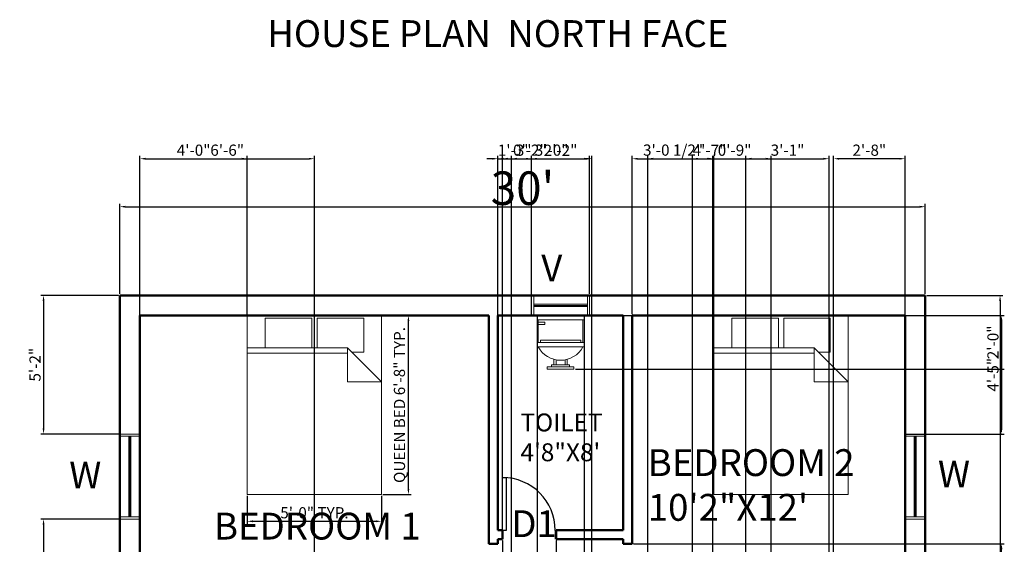
# Model space of a CAD drawing. Units: inches. Extents: x 2050 to 2529, y 1266 to 1968.
# Tile 5 of 5: x 2050 to 2490, y 1733 to 1968. Entities that reach past the tile are written whole.
import ezdxf

# ---------------------------------------------------------------- set-up
doc = ezdxf.new("R2010")
doc.units = ezdxf.units.IN
for name, color, linetype, lineweight in [('A-ANNO-DIMS', 2, 'Continuous', 18), ('A-ANNO-TEXT', 7, 'Continuous', 18), ('A-AREA-IDEN', 7, 'Continuous', 25), ('A-DOOR', 3, 'Continuous', 25), ('A-FLOR-FIXT', 9, 'Continuous', 18), ('A-FURN', 8, 'Continuous', 18), ('A-GLAZ', 4, 'Continuous', 18), ('A-WALL', 7, 'Continuous', 50)]:
    doc.layers.add(name, color=color, linetype=linetype, lineweight=lineweight)
doc.styles.get("Standard").update_dxf_attribs({"font": 'arial.ttf'})
doc.dimstyles.new('ISO-25', dxfattribs={"dimtxt": 5, "dimasz": 2.5, "dimexe": 1.25, "dimexo": 0.625, "dimtad": 1, "dimlunit": 3, "dimtxsty": 'Standard', "dimcen": 2.5, "dimadec": 0, "dimazin": 0, "dimtfac": 1, "dimtmove": 0, "dimatfit": 3, "dimfxl": 1, "dimarcsym": 0})

# ---------------------------------------------------------------- blocks, each defined once
blk = doc.blocks.new('*D1')
at = {"layer": 'A-ANNO-DIMS', "color": 0, "lineweight": -2, "transparency": 16777216}
for p, q in [((2094.29, 1845.35), (2094.29, 1885.6)), ((2096.79, 1884.35), (2451.79, 1884.35)), ((2454.29, 1845.35), (2454.29, 1885.6))]:
    blk.add_line(p, q, dxfattribs=at)
at = {"layer": 'A-ANNO-DIMS', "color": 0, "transparency": 16777216}
for points in [[(2096.79, 1884.76), (2096.79, 1883.93), (2094.29, 1884.35)], [(2451.79, 1884.76), (2451.79, 1883.93), (2454.29, 1884.35)]]:
    blk.add_solid(points, dxfattribs=at)
at = {"layer": 'Defpoints', "color": 0, "transparency": 16777216}
for p in [(2454.29, 1884.35), (2094.29, 1844.72), (2454.29, 1844.72)]:
    blk.add_point(p, dxfattribs=at)
at = {"layer": 'A-ANNO-DIMS', "color": 0, "transparency": 16777216, "insert": (2274.29, 1892.63), "char_height": 5, "attachment_point": 5}
blk.add_mtext("{\\H3x;30'}", dxfattribs=at)
blk = doc.blocks.new('*D2')
at = {"layer": 'A-ANNO-DIMS', "color": 0, "lineweight": -2, "transparency": 16777216}
for p, q in [((2454.92, 1844.72), (2488.97, 1844.72)), ((2487.72, 1842.22), (2487.72, 1307.22)), ((2454.92, 1304.72), (2488.97, 1304.72))]:
    blk.add_line(p, q, dxfattribs=at)
at = {"layer": 'A-ANNO-DIMS', "color": 0, "transparency": 16777216}
for points in [[(2487.3, 1842.22), (2488.13, 1842.22), (2487.72, 1844.72)], [(2487.3, 1307.22), (2488.13, 1307.22), (2487.72, 1304.72)]]:
    blk.add_solid(points, dxfattribs=at)
at = {"layer": 'Defpoints', "color": 0, "transparency": 16777216}
for p in [(2454.29, 1844.72), (2454.29, 1304.72), (2487.72, 1304.72)]:
    blk.add_point(p, dxfattribs=at)
at = {"layer": 'A-ANNO-DIMS', "color": 0, "transparency": 16777216, "insert": (2479.46, 1574.72), "char_height": 5, "attachment_point": 5, "rotation": 90}
blk.add_mtext("{\\H3x;45'}", dxfattribs=at)
blk = doc.blocks.new('*U8')
for p, q in [((0, 0), (0, -100)), ((600, 0), (600, -100))]:
    blk.add_line(p, q)
blk.add_lwpolyline([(0, 0), (0, 600), (43.75, 600), (43.75, 0)], close=True)
blk.add_arc((0, 0), 600, 0, 90)
blk = doc.blocks.new('Bed - Queen')
for p, q in [((0, -80.00003), (0, 0)), ((0, 0), (59.99999, 0)), ((59.99999, 0), (59.99999, -80.00003)), ((7.99999, -1.2), (28.79998, -1.2)), ((7.99999, -14.4), (7.99999, -1.2)), ((28.79998, -1.2), (28.79998, -14.4)), ((31.19999, -1.2), (51.99999, -1.2)), ((31.19999, -14.4), (31.19999, -1.2)), ((51.99999, -1.2), (51.99999, -16.4)), ((0, -14.4), (44.8, -14.4)), ((44.8, -16.8), (0, -16.8)), ((59.99999, -29.6), (44.8, -14.4)), ((44.8, -14.4), (44.8, -29.6)), ((51.99999, -16.4), (46.79936, -16.4)), ((44.8, -29.6), (59.99999, -29.6)), ((59.99999, -80.00003), (0, -80.00003))]:
    blk.add_line(p, q)
blk = doc.blocks.new('*U13')
for p, q in [((-254, 558.8), (-254, 304.8)), ((-254, 533.4), (-177.8, 533.4)), ((-177.8, 508), (-254, 508)), ((-177.8, 533.4), (-177.8, 508)), ((254, 304.8), (254, 558.8)), ((266.7, 304.8), (-266.7, 304.8)), ((-266.7, 254), (-266.7, 304.8)), ((266.7, 254), (-266.7, 254)), ((228.6, 330.2), (-228.6, 330.2)), ((-228.6, 330.2), (-228.6, 304.8)), ((228.6, 304.8), (228.6, 330.2)), ((266.7, 304.8), (266.7, 254)), ((-76.2, 111.9251), (-76.2, 50.8)), ((76.2, 50.8), (76.2, 111.9251)), ((101.6, 50.8), (-101.6, 50.8)), ((-101.6, 50.8), (-101.6, 25.4)), ((-50.8, 50.8), (-50.8, 105.81132)), ((50.8, 105.81132), (50.8, 50.8)), ((101.6, 25.4), (101.6, 50.8))]:
    blk.add_line(p, q)
for points in [[(266.7, 558.8), (266.7, 609.6), (-266.7, 609.6), (-266.7, 558.8)], [(152.4, 0), (152.4, 25.4), (-152.4, 25.4), (-152.4, 0)]]:
    blk.add_lwpolyline(points, close=True)
blk.add_arc((0, 389.46582), 287.86658, 208.0725, 331.9275)
blk = doc.blocks.new('WIN-36IN')
for p, q in [((0, 9), (0, 0)), ((1, 9), (1, 0)), ((37, 9), (37, 0)), ((38, 9), (38, 0)), ((1, 5), (37, 5)), ((1, 4.5), (37, 4.5)), ((1, 4), (37, 4))]:
    blk.add_line(p, q)
blk = doc.blocks.new('*D28')
at = {"layer": 'A-ANNO-DIMS', "color": 0, "lineweight": -2, "transparency": 16777216}
for p, q in [((2211.92, 1835.72), (2224.54, 1835.72)), ((2223.29, 1758.22), (2223.29, 1833.22)), ((2211.92, 1755.72), (2224.54, 1755.72))]:
    blk.add_line(p, q, dxfattribs=at)
at = {"layer": 'A-ANNO-DIMS', "color": 0, "transparency": 16777216}
for points in [[(2222.88, 1833.22), (2223.71, 1833.22), (2223.29, 1835.72)], [(2222.88, 1758.22), (2223.71, 1758.22), (2223.29, 1755.72)]]:
    blk.add_solid(points, dxfattribs=at)
at = {"layer": 'Defpoints', "color": 0, "transparency": 16777216}
for p in [(2211.29, 1835.72), (2223.29, 1835.72), (2211.29, 1755.72)]:
    blk.add_point(p, dxfattribs=at)
at = {"layer": 'A-ANNO-DIMS', "color": 0, "transparency": 16777216, "insert": (2219.93, 1795.72), "char_height": 5, "attachment_point": 5, "rotation": 90}
blk.add_mtext('QUEEN BED 6\'-8" TYP.', dxfattribs=at)
blk = doc.blocks.new('*D29')
at = {"layer": 'A-ANNO-DIMS', "color": 0, "lineweight": -2, "transparency": 16777216}
for p, q in [((2151.29, 1755.1), (2151.29, 1742.47)), ((2211.29, 1755.1), (2211.29, 1742.47)), ((2153.79, 1743.72), (2208.79, 1743.72))]:
    blk.add_line(p, q, dxfattribs=at)
at = {"layer": 'A-ANNO-DIMS', "color": 0, "transparency": 16777216}
for points in [[(2153.79, 1744.14), (2153.79, 1743.3), (2151.29, 1743.72)], [(2208.79, 1744.14), (2208.79, 1743.3), (2211.29, 1743.72)]]:
    blk.add_solid(points, dxfattribs=at)
at = {"layer": 'Defpoints', "color": 0, "transparency": 16777216}
for p in [(2151.29, 1755.72), (2211.29, 1755.72), (2211.29, 1743.72)]:
    blk.add_point(p, dxfattribs=at)
at = {"layer": 'A-ANNO-DIMS', "color": 0, "transparency": 16777216, "insert": (2181.29, 1746.9), "char_height": 5, "attachment_point": 5}
blk.add_mtext('5\'-0" TYP.', dxfattribs=at)
blk = doc.blocks.new('*D43')
at = {"layer": 'A-ANNO-DIMS', "color": 0, "lineweight": -2, "transparency": 16777216}
for p, q in [((2103.29, 1686.35), (2103.29, 1907.05)), ((2105.79, 1905.8), (2178.79, 1905.8)), ((2181.29, 1686.35), (2181.29, 1907.05))]:
    blk.add_line(p, q, dxfattribs=at)
at = {"layer": 'A-ANNO-DIMS', "color": 0, "transparency": 16777216}
for points in [[(2105.79, 1906.21), (2105.79, 1905.38), (2103.29, 1905.8)], [(2178.79, 1906.21), (2178.79, 1905.38), (2181.29, 1905.8)]]:
    blk.add_solid(points, dxfattribs=at)
at = {"layer": 'Defpoints', "color": 0, "transparency": 16777216}
for p in [(2181.29, 1905.8), (2103.29, 1685.72), (2181.29, 1685.72)]:
    blk.add_point(p, dxfattribs=at)
at = {"layer": 'A-ANNO-DIMS', "color": 0, "transparency": 16777216, "insert": (2142.29, 1908.97), "char_height": 5, "attachment_point": 5}
blk.add_mtext('6\'-6"', dxfattribs=at)
blk = doc.blocks.new('*D51')
at = {"layer": 'A-ANNO-DIMS', "color": 0, "lineweight": -2, "transparency": 16777216}
for p, q in [((2413.29, 1314.35), (2413.29, 1907.05)), ((2442.79, 1905.8), (2415.79, 1905.8)), ((2445.29, 1314.35), (2445.29, 1907.05))]:
    blk.add_line(p, q, dxfattribs=at)
at = {"layer": 'A-ANNO-DIMS', "color": 0, "transparency": 16777216}
for points in [[(2415.79, 1906.21), (2415.79, 1905.38), (2413.29, 1905.8)], [(2442.79, 1906.21), (2442.79, 1905.38), (2445.29, 1905.8)]]:
    blk.add_solid(points, dxfattribs=at)
at = {"layer": 'Defpoints', "color": 0, "transparency": 16777216}
for p in [(2413.29, 1905.8), (2413.29, 1313.72), (2445.29, 1313.72)]:
    blk.add_point(p, dxfattribs=at)
at = {"layer": 'A-ANNO-DIMS', "color": 0, "transparency": 16777216, "insert": (2429.29, 1908.97), "char_height": 5, "attachment_point": 5}
blk.add_mtext('2\'-8"', dxfattribs=at)
blk = doc.blocks.new('*D52')
at = {"layer": 'A-ANNO-DIMS', "color": 0, "lineweight": -2, "transparency": 16777216}
for p, q in [((2350.29, 1390.35), (2350.29, 1907.05)), ((2352.79, 1905.8), (2356.79, 1905.8)), ((2359.29, 1390.35), (2359.29, 1907.05)), ((2359.29, 1905.8), (2376.34, 1905.8))]:
    blk.add_line(p, q, dxfattribs=at)
at = {"layer": 'A-ANNO-DIMS', "color": 0, "transparency": 16777216}
for points in [[(2352.79, 1906.21), (2352.79, 1905.38), (2350.29, 1905.8)], [(2356.79, 1906.21), (2356.79, 1905.38), (2359.29, 1905.8)]]:
    blk.add_solid(points, dxfattribs=at)
at = {"layer": 'Defpoints', "color": 0, "transparency": 16777216}
for p in [(2359.29, 1905.8), (2350.29, 1389.72), (2359.29, 1389.72)]:
    blk.add_point(p, dxfattribs=at)
at = {"layer": 'A-ANNO-DIMS', "color": 0, "transparency": 16777216, "insert": (2369.07, 1908.97), "char_height": 5, "attachment_point": 5}
blk.add_mtext('0\'-9"', dxfattribs=at)
blk = doc.blocks.new('*D54')
at = {"layer": 'A-ANNO-DIMS', "color": 0, "lineweight": -2, "transparency": 16777216}
for p, q in [((2269.29, 1396.35), (2269.29, 1907.05)), ((2271.79, 1905.8), (2302.79, 1905.8)), ((2305.29, 1396.35), (2305.29, 1907.05))]:
    blk.add_line(p, q, dxfattribs=at)
at = {"layer": 'A-ANNO-DIMS', "color": 0, "transparency": 16777216}
for points in [[(2271.79, 1906.21), (2271.79, 1905.38), (2269.29, 1905.8)], [(2302.79, 1906.21), (2302.79, 1905.38), (2305.29, 1905.8)]]:
    blk.add_solid(points, dxfattribs=at)
at = {"layer": 'Defpoints', "color": 0, "transparency": 16777216}
for p in [(2305.29, 1905.8), (2269.29, 1395.72), (2305.29, 1395.72)]:
    blk.add_point(p, dxfattribs=at)
at = {"layer": 'A-ANNO-DIMS', "color": 0, "transparency": 16777216, "insert": (2287.29, 1908.98), "char_height": 5, "attachment_point": 5}
blk.add_mtext('3\'-0"', dxfattribs=at)
blk = doc.blocks.new('*D56')
at = {"layer": 'A-ANNO-DIMS', "color": 0, "lineweight": -2, "transparency": 16777216}
for p, q in [((2323.92, 1733.72), (2489.62, 1733.72)), ((2488.37, 1700.22), (2488.37, 1731.22)), ((2323.92, 1697.72), (2489.62, 1697.72))]:
    blk.add_line(p, q, dxfattribs=at)
at = {"layer": 'A-ANNO-DIMS', "color": 0, "transparency": 16777216}
for points in [[(2487.95, 1731.22), (2488.79, 1731.22), (2488.37, 1733.72)], [(2487.95, 1700.22), (2488.79, 1700.22), (2488.37, 1697.72)]]:
    blk.add_solid(points, dxfattribs=at)
at = {"layer": 'Defpoints', "color": 0, "transparency": 16777216}
for p in [(2323.29, 1733.72), (2488.37, 1733.72), (2323.29, 1697.72)]:
    blk.add_point(p, dxfattribs=at)
at = {"layer": 'A-ANNO-DIMS', "color": 0, "transparency": 16777216, "insert": (2485.19, 1715.72), "char_height": 5, "attachment_point": 5, "rotation": 90}
blk.add_mtext('3\'-0"', dxfattribs=at)
blk = doc.blocks.new('*D60')
at = {"layer": 'A-ANNO-DIMS', "color": 0, "lineweight": -2, "transparency": 16777216}
for p, q in [((2265.29, 1735.1), (2265.29, 1269.4)), ((2289.29, 1735.1), (2289.29, 1269.4)), ((2267.79, 1270.65), (2286.79, 1270.65))]:
    blk.add_line(p, q, dxfattribs=at)
at = {"layer": 'A-ANNO-DIMS', "color": 0, "transparency": 16777216}
for points in [[(2267.79, 1271.06), (2267.79, 1270.23), (2265.29, 1270.65)], [(2286.79, 1271.06), (2286.79, 1270.23), (2289.29, 1270.65)]]:
    blk.add_solid(points, dxfattribs=at)
at = {"layer": 'Defpoints', "color": 0, "transparency": 16777216}
for p in [(2265.29, 1735.72), (2289.29, 1735.72), (2289.29, 1270.65)]:
    blk.add_point(p, dxfattribs=at)
at = {"layer": 'A-ANNO-DIMS', "color": 0, "transparency": 16777216, "insert": (2277.29, 1273.82), "char_height": 5, "attachment_point": 5}
blk.add_mtext('2\'-0"', dxfattribs=at)
blk = doc.blocks.new('*D61')
at = {"layer": 'A-ANNO-DIMS', "color": 0, "lineweight": -2, "transparency": 16777216}
for p, q in [((2260.79, 1905.8), (2258.29, 1905.8)), ((2263.29, 1740.35), (2263.29, 1907.05)), ((2263.29, 1905.8), (2265.29, 1905.8)), ((2265.29, 1740.35), (2265.29, 1907.05)), ((2267.79, 1905.8), (2284.84, 1905.8))]:
    blk.add_line(p, q, dxfattribs=at)
at = {"layer": 'A-ANNO-DIMS', "color": 0, "transparency": 16777216}
for points in [[(2260.79, 1906.21), (2260.79, 1905.38), (2263.29, 1905.8)], [(2267.79, 1906.21), (2267.79, 1905.38), (2265.29, 1905.8)]]:
    blk.add_solid(points, dxfattribs=at)
at = {"layer": 'Defpoints', "color": 0, "transparency": 16777216}
for p in [(2265.29, 1905.8), (2263.29, 1739.72), (2265.29, 1739.72)]:
    blk.add_point(p, dxfattribs=at)
at = {"layer": 'A-ANNO-DIMS', "color": 0, "transparency": 16777216, "insert": (2277.57, 1908.97), "char_height": 5, "attachment_point": 5}
blk.add_mtext('0\'-2"', dxfattribs=at)
blk = doc.blocks.new('*D62')
at = {"layer": 'A-ANNO-DIMS', "color": 0, "lineweight": -2, "transparency": 16777216}
for p, q in [((2278.29, 1845.35), (2278.29, 1907.05)), ((2280.79, 1905.8), (2301.79, 1905.8)), ((2304.29, 1845.35), (2304.29, 1907.05))]:
    blk.add_line(p, q, dxfattribs=at)
at = {"layer": 'A-ANNO-DIMS', "color": 0, "transparency": 16777216}
for points in [[(2280.79, 1906.21), (2280.79, 1905.38), (2278.29, 1905.8)], [(2301.79, 1906.21), (2301.79, 1905.38), (2304.29, 1905.8)]]:
    blk.add_solid(points, dxfattribs=at)
at = {"layer": 'Defpoints', "color": 0, "transparency": 16777216}
for p in [(2304.29, 1905.8), (2278.29, 1844.72), (2304.29, 1844.72)]:
    blk.add_point(p, dxfattribs=at)
at = {"layer": 'A-ANNO-DIMS', "color": 0, "transparency": 16777216, "insert": (2291.29, 1908.93), "char_height": 5, "attachment_point": 5}
blk.add_mtext('2\'-2"', dxfattribs=at)
blk = doc.blocks.new('*D63')
at = {"layer": 'A-ANNO-DIMS', "color": 0, "lineweight": -2, "transparency": 16777216}
for p, q in [((2263.29, 1836.35), (2263.29, 1907.05)), ((2265.79, 1905.8), (2275.79, 1905.8)), ((2278.29, 1836.35), (2278.29, 1907.05))]:
    blk.add_line(p, q, dxfattribs=at)
at = {"layer": 'A-ANNO-DIMS', "color": 0, "transparency": 16777216}
for points in [[(2265.79, 1906.21), (2265.79, 1905.38), (2263.29, 1905.8)], [(2275.79, 1906.21), (2275.79, 1905.38), (2278.29, 1905.8)]]:
    blk.add_solid(points, dxfattribs=at)
at = {"layer": 'Defpoints', "color": 0, "transparency": 16777216}
for p in [(2278.29, 1905.8), (2263.29, 1835.72), (2278.29, 1835.72)]:
    blk.add_point(p, dxfattribs=at)
at = {"layer": 'A-ANNO-DIMS', "color": 0, "transparency": 16777216, "insert": (2270.79, 1908.98), "char_height": 5, "attachment_point": 5}
blk.add_mtext('1\'-3"', dxfattribs=at)
blk = doc.blocks.new('*D64')
at = {"layer": 'A-ANNO-DIMS', "color": 0, "lineweight": -2, "transparency": 16777216}
for p, q in [((2280.79, 1835.1), (2280.79, 1269.4)), ((2301.79, 1835.1), (2301.79, 1269.4)), ((2283.29, 1270.65), (2299.29, 1270.65))]:
    blk.add_line(p, q, dxfattribs=at)
at = {"layer": 'A-ANNO-DIMS', "color": 0, "transparency": 16777216}
for points in [[(2283.29, 1271.06), (2283.29, 1270.23), (2280.79, 1270.65)], [(2299.29, 1271.06), (2299.29, 1270.23), (2301.79, 1270.65)]]:
    blk.add_solid(points, dxfattribs=at)
at = {"layer": 'Defpoints', "color": 0, "transparency": 16777216}
for p in [(2280.79, 1835.72), (2301.79, 1835.72), (2301.79, 1270.65)]:
    blk.add_point(p, dxfattribs=at)
at = {"layer": 'A-ANNO-DIMS', "color": 0, "transparency": 16777216, "insert": (2291.29, 1273.82), "char_height": 5, "attachment_point": 5}
blk.add_mtext('1\'-9"', dxfattribs=at)
blk = doc.blocks.new('*D65')
at = {"layer": 'A-ANNO-DIMS', "color": 0, "lineweight": -2, "transparency": 16777216}
for p, q in [((2302.42, 1835.72), (2489.62, 1835.72)), ((2488.37, 1814.22), (2488.37, 1833.22)), ((2297.92, 1811.72), (2489.62, 1811.72))]:
    blk.add_line(p, q, dxfattribs=at)
at = {"layer": 'A-ANNO-DIMS', "color": 0, "transparency": 16777216}
for points in [[(2487.95, 1833.22), (2488.79, 1833.22), (2488.37, 1835.72)], [(2487.95, 1814.22), (2488.79, 1814.22), (2488.37, 1811.72)]]:
    blk.add_solid(points, dxfattribs=at)
at = {"layer": 'Defpoints', "color": 0, "transparency": 16777216}
for p in [(2301.79, 1835.72), (2488.37, 1835.72), (2297.29, 1811.72)]:
    blk.add_point(p, dxfattribs=at)
at = {"layer": 'A-ANNO-DIMS', "color": 0, "transparency": 16777216, "insert": (2485.19, 1823.72), "char_height": 5, "attachment_point": 5, "rotation": 90}
blk.add_mtext('2\'-0"', dxfattribs=at)
blk = doc.blocks.new('*D66')
at = {"layer": 'A-ANNO-DIMS', "color": 0, "lineweight": -2, "transparency": 16777216}
for p, q in [((2093.67, 1844.72), (2058.97, 1844.72)), ((2060.22, 1842.22), (2060.22, 1785.22)), ((2093.67, 1782.72), (2058.97, 1782.72))]:
    blk.add_line(p, q, dxfattribs=at)
at = {"layer": 'A-ANNO-DIMS', "color": 0, "transparency": 16777216}
for points in [[(2059.8, 1842.22), (2060.64, 1842.22), (2060.22, 1844.72)], [(2059.8, 1785.22), (2060.64, 1785.22), (2060.22, 1782.72)]]:
    blk.add_solid(points, dxfattribs=at)
at = {"layer": 'Defpoints', "color": 0, "transparency": 16777216}
for p in [(2094.29, 1844.72), (2060.22, 1782.72), (2094.29, 1782.72)]:
    blk.add_point(p, dxfattribs=at)
at = {"layer": 'A-ANNO-DIMS', "color": 0, "transparency": 16777216, "insert": (2057.04, 1813.72), "char_height": 5, "attachment_point": 5, "rotation": 90}
blk.add_mtext('5\'-2"', dxfattribs=at)
blk = doc.blocks.new('*D67')
at = {"layer": 'A-ANNO-DIMS', "color": 0, "lineweight": -2, "transparency": 16777216}
for p, q in [((2093.67, 1744.72), (2058.97, 1744.72)), ((2060.22, 1742.22), (2060.22, 1657.72)), ((2093.67, 1655.22), (2058.97, 1655.22))]:
    blk.add_line(p, q, dxfattribs=at)
at = {"layer": 'A-ANNO-DIMS', "color": 0, "transparency": 16777216}
for points in [[(2059.8, 1742.22), (2060.64, 1742.22), (2060.22, 1744.72)], [(2059.8, 1657.72), (2060.64, 1657.72), (2060.22, 1655.22)]]:
    blk.add_solid(points, dxfattribs=at)
at = {"layer": 'Defpoints', "color": 0, "transparency": 16777216}
for p in [(2094.29, 1744.72), (2060.22, 1655.22), (2094.29, 1655.22)]:
    blk.add_point(p, dxfattribs=at)
at = {"layer": 'A-ANNO-DIMS', "color": 0, "transparency": 16777216, "insert": (2057.01, 1699.97), "char_height": 5, "attachment_point": 5, "rotation": 90}
blk.add_mtext('7\'-5 1/2"', dxfattribs=at)
blk = doc.blocks.new('*D70')
at = {"layer": 'A-ANNO-DIMS', "color": 0, "lineweight": -2, "transparency": 16777216}
for p, q in [((2445.92, 1835.72), (2489.62, 1835.72)), ((2488.37, 1833.22), (2488.37, 1785.22)), ((2445.92, 1782.72), (2489.62, 1782.72))]:
    blk.add_line(p, q, dxfattribs=at)
at = {"layer": 'A-ANNO-DIMS', "color": 0, "transparency": 16777216}
for points in [[(2487.95, 1833.22), (2488.79, 1833.22), (2488.37, 1835.72)], [(2487.95, 1785.22), (2488.79, 1785.22), (2488.37, 1782.72)]]:
    blk.add_solid(points, dxfattribs=at)
at = {"layer": 'Defpoints', "color": 0, "transparency": 16777216}
for p in [(2445.29, 1835.72), (2445.29, 1782.72), (2488.37, 1782.72)]:
    blk.add_point(p, dxfattribs=at)
at = {"layer": 'A-ANNO-DIMS', "color": 0, "transparency": 16777216, "insert": (2485.2, 1809.22), "char_height": 5, "attachment_point": 5, "rotation": 90}
blk.add_mtext('4\'-5"', dxfattribs=at)
blk = doc.blocks.new('*D74')
at = {"layer": 'A-ANNO-DIMS', "color": 0, "lineweight": -2, "transparency": 16777216}
for p, q in [((2103.29, 1836.35), (2103.29, 1907.05)), ((2105.79, 1905.8), (2148.79, 1905.8)), ((2151.29, 1836.35), (2151.29, 1907.05))]:
    blk.add_line(p, q, dxfattribs=at)
at = {"layer": 'A-ANNO-DIMS', "color": 0, "transparency": 16777216}
for points in [[(2105.79, 1906.21), (2105.79, 1905.38), (2103.29, 1905.8)], [(2148.79, 1906.21), (2148.79, 1905.38), (2151.29, 1905.8)]]:
    blk.add_solid(points, dxfattribs=at)
at = {"layer": 'Defpoints', "color": 0, "transparency": 16777216}
for p in [(2151.29, 1905.8), (2103.29, 1835.72), (2151.29, 1835.72)]:
    blk.add_point(p, dxfattribs=at)
at = {"layer": 'A-ANNO-DIMS', "color": 0, "transparency": 16777216, "insert": (2127.29, 1908.97), "char_height": 5, "attachment_point": 5}
blk.add_mtext('4\'-0"', dxfattribs=at)
blk = doc.blocks.new('*D75')
at = {"layer": 'A-ANNO-DIMS', "color": 0, "lineweight": -2, "transparency": 16777216}
for p, q in [((2323.29, 1836.35), (2323.29, 1907.05)), ((2325.79, 1905.8), (2357.36, 1905.8)), ((2359.86, 1836.35), (2359.86, 1907.05))]:
    blk.add_line(p, q, dxfattribs=at)
at = {"layer": 'A-ANNO-DIMS', "color": 0, "transparency": 16777216}
for points in [[(2325.79, 1906.21), (2325.79, 1905.38), (2323.29, 1905.8)], [(2357.36, 1906.21), (2357.36, 1905.38), (2359.86, 1905.8)]]:
    blk.add_solid(points, dxfattribs=at)
at = {"layer": 'Defpoints', "color": 0, "transparency": 16777216}
for p in [(2359.86, 1905.8), (2323.29, 1835.72), (2359.86, 1835.72)]:
    blk.add_point(p, dxfattribs=at)
at = {"layer": 'A-ANNO-DIMS', "color": 0, "transparency": 16777216, "insert": (2341.58, 1909.01), "char_height": 5, "attachment_point": 5}
blk.add_mtext('3\'-0 1/2"', dxfattribs=at)
blk = doc.blocks.new('*D77')
at = {"layer": 'A-ANNO-DIMS', "color": 0, "lineweight": -2, "transparency": 16777216}
for p, q in [((2330.24, 1637.61), (2330.24, 1907.05)), ((2332.74, 1905.8), (2382.97, 1905.8)), ((2385.47, 1637.61), (2385.47, 1907.05))]:
    blk.add_line(p, q, dxfattribs=at)
at = {"layer": 'A-ANNO-DIMS', "color": 0, "transparency": 16777216}
for points in [[(2332.74, 1906.21), (2332.74, 1905.38), (2330.24, 1905.8)], [(2382.97, 1906.21), (2382.97, 1905.38), (2385.47, 1905.8)]]:
    blk.add_solid(points, dxfattribs=at)
at = {"layer": 'Defpoints', "color": 0, "transparency": 16777216}
for p in [(2385.47, 1905.8), (2330.24, 1636.98), (2385.47, 1636.98)]:
    blk.add_point(p, dxfattribs=at)
at = {"layer": 'A-ANNO-DIMS', "color": 0, "transparency": 16777216, "insert": (2357.86, 1908.92), "char_height": 5, "attachment_point": 5}
blk.add_mtext('4\'-7"', dxfattribs=at)
blk = doc.blocks.new('*D79')
at = {"layer": 'A-ANNO-DIMS', "color": 0, "lineweight": -2, "transparency": 16777216}
for p, q in [((2374.17, 1568.26), (2374.17, 1907.05)), ((2376.67, 1905.8), (2408.79, 1905.8)), ((2411.29, 1583.35), (2411.29, 1907.05))]:
    blk.add_line(p, q, dxfattribs=at)
at = {"layer": 'A-ANNO-DIMS', "color": 0, "transparency": 16777216}
for points in [[(2376.67, 1906.21), (2376.67, 1905.38), (2374.17, 1905.8)], [(2408.79, 1906.21), (2408.79, 1905.38), (2411.29, 1905.8)]]:
    blk.add_solid(points, dxfattribs=at)
at = {"layer": 'Defpoints', "color": 0, "transparency": 16777216}
for p in [(2411.29, 1905.8), (2411.29, 1582.72), (2374.17, 1567.64)]:
    blk.add_point(p, dxfattribs=at)
at = {"layer": 'A-ANNO-DIMS', "color": 0, "transparency": 16777216, "insert": (2392.73, 1908.98), "char_height": 5, "attachment_point": 5}
blk.add_mtext('3\'-1"', dxfattribs=at)

msp = doc.modelspace()

# ---------------------------------------------------------------- linework, layer by layer
at = {"layer": 'A-GLAZ'}
for p, q in [((2278.295, 1844.72), (2278.295, 1835.72)), ((2279.295, 1844.72), (2279.295, 1835.72)), ((2303.295, 1844.72), (2303.295, 1835.72)), ((2304.295, 1844.72), (2304.295, 1835.72)), ((2279.295, 1840.72), (2303.295, 1840.72)), ((2279.295, 1840.22), (2303.295, 1840.22)), ((2279.295, 1839.72), (2303.295, 1839.72))]:
    msp.add_line(p, q, dxfattribs=at)
at = {"layer": 'A-WALL'}
for p, q in [((2094.295, 1844.72), (2454.295, 1844.72)), ((2094.295, 1304.72), (2094.295, 1844.72)), ((2454.295, 1844.72), (2454.295, 1304.72)), ((2103.295, 1835.72), (2259.295, 1835.72)), ((2103.295, 1691.72), (2103.295, 1835.72)), ((2259.295, 1733.72), (2259.295, 1835.72)), ((2263.295, 1739.72), (2263.295, 1835.72)), ((2263.295, 1835.72), (2319.295, 1835.72)), ((2319.295, 1739.72), (2319.295, 1835.72)), ((2323.295, 1733.72), (2323.295, 1835.72)), ((2323.295, 1835.72), (2445.295, 1835.72)), ((2445.295, 1835.72), (2445.295, 1691.72)), ((2263.295, 1739.72), (2265.295, 1739.72)), ((2265.295, 1739.72), (2265.295, 1735.72)), ((2289.295, 1739.72), (2289.295, 1735.72)), ((2289.295, 1739.72), (2319.295, 1739.72)), ((2263.295, 1735.72), (2265.295, 1735.72)), ((2263.295, 1733.72), (2263.295, 1735.72)), ((2289.295, 1735.72), (2319.295, 1735.72)), ((2319.295, 1733.72), (2319.295, 1735.72)), ((2259.295, 1733.72), (2263.295, 1733.72)), ((2319.295, 1733.72), (2323.295, 1733.72))]:
    msp.add_line(p, q, dxfattribs=at)

# ---------------------------------------------------------------- block references
at = {"layer": 'A-DOOR', "xscale": 0.0393700787401575, "yscale": 0.0393700787401575, "zscale": 0.0393700787401575}
msp.add_blockref('*U8', (2265.295, 1739.657), dxfattribs=at)
at = {"layer": 'A-FLOR-FIXT', "xscale": 0.0393700787401575, "yscale": 0.0393700787401575, "zscale": 0.0393700787401575}
msp.add_blockref('*U13', (2291.295, 1811.72), dxfattribs=at)
at = {"layer": 'A-FURN'}
for p in [(2151.295, 1835.72), (2359.858, 1835.72)]:
    msp.add_blockref('Bed - Queen', p, dxfattribs=at)
at = {"layer": 'A-GLAZ'}
for p, rotation in [((2094.294, 1782.72), 269.999999999998), ((2445.294, 1782.72), 269.9999999999999)]:
    msp.add_blockref('WIN-36IN', p, dxfattribs=dict(at, rotation=rotation))

# ---------------------------------------------------------------- texts
at = {"layer": 'A-ANNO-TEXT', "char_height": 12, "attachment_point": 1}
for s, width, heights, insert in [('HOUSE PLAN  NORTH FACE', 649.2389, [75.088], (2160.186, 1967.737)), ('V', 471.52273, [28.462], (2282.66, 1862.953)), ('W', 471.52273, [28.462], (2071.678, 1770.45)), ('W', 471.52273, [28.462], (2459.945, 1770.866)), ('D1', 471.52273, [28.462], (2269.295, 1748.642))]:
    msp.add_mtext_dynamic_manual_height_columns(s, width=width, gutter_width=12.5, heights=heights, dxfattribs=dict(at, insert=insert))
at = {"layer": 'A-AREA-IDEN', "attachment_point": 1}
for s, insert, char_height in [('TOILET\\P4\'8"X8\'', (2273.368, 1791.91), 8), ('BEDROOM 2\\P10\'2"X12\'', (2330.265, 1775.955), 12), ("BEDROOM 1\\P13'X12'", (2136.374, 1747.567), 12)]:
    msp.add_mtext_dynamic_manual_height_columns(s, width=649.2389, gutter_width=12.5, heights=[75.088], dxfattribs=dict(at, insert=insert, char_height=char_height))

# ---------------------------------------------------------------- dimensions: what is measured, and where the dimension line sits
at = {"layer": 'A-ANNO-DIMS'}
for base, p1, p2, picture, middle in [((2359.858, 1905.795), (2323.295, 1835.72), (2359.858, 1835.72), '*D75', (2341.577, 1909.007)), ((2181.295, 1905.795), (2103.295, 1685.72), (2181.295, 1685.72), '*D43', (2142.295, 1908.973)), ((2151.295, 1905.795), (2103.295, 1835.72), (2151.295, 1835.72), '*D74', (2127.295, 1908.973)), ((2265.295, 1905.795), (2263.295, 1739.72), (2265.295, 1739.72), '*D61', (2277.565, 1908.973)), ((2278.295, 1905.795), (2263.295, 1835.72), (2278.295, 1835.72), '*D63', (2270.795, 1908.975)), ((2305.295, 1905.795), (2269.295, 1395.72), (2305.295, 1395.72), '*D54', (2287.295, 1908.975)), ((2304.295, 1905.795), (2278.295, 1844.72), (2304.295, 1844.72), '*D62', (2291.295, 1908.931)), ((2385.471, 1905.795), (2330.24, 1636.982), (2385.471, 1636.982), '*D77', (2357.856, 1908.92)), ((2359.295, 1905.795), (2350.295, 1389.72), (2359.295, 1389.72), '*D52', (2369.065, 1908.973)), ((2411.295, 1905.795), (2374.175, 1567.637), (2411.295, 1582.72), '*D79', (2392.735, 1908.975)), ((2413.295, 1905.795), (2445.295, 1313.72), (2413.295, 1313.72), '*D51', (2429.295, 1908.973)), ((2301.795, 1270.645), (2280.795, 1835.72), (2301.795, 1835.72), '*D64', (2291.295, 1273.823)), ((2289.295, 1270.645), (2265.295, 1735.72), (2289.295, 1735.72), '*D60', (2277.295, 1273.823))]:
    dim = msp.add_linear_dim(base=base, p1=p1, p2=p2, dimstyle='ISO-25', override={"dimdec": 1, "dimlfac": 1, "dimrnd": 0, "dimzin": 1, "dimdsep": 46, "dimlunit": 4, "dimfrac": 2}, dxfattribs=at)
    dim.commit()
    dim.dimension.update_dxf_attribs({"geometry": picture, "text_midpoint": middle})
for base, p1, p2, text, override, picture, middle in [((2454.295, 1884.345), (2094.295, 1844.72), (2454.295, 1844.72), '{\\H3x;<>}', {"dimclrd": 0, "dimclre": 0, "dimclrt": 0}, '*D1', (2274.295, 1892.634)), ((2211.295, 1743.72), (2151.295, 1755.72), (2211.295, 1755.72), '<> TYP.', {"dimdec": 1, "dimlfac": 1, "dimrnd": 0, "dimzin": 1, "dimdsep": 46, "dimlunit": 4, "dimfrac": 2}, '*D29', (2181.295, 1746.898))]:
    dim = msp.add_linear_dim(base=base, p1=p1, p2=p2, text=text, dimstyle='ISO-25', override=override, dxfattribs=at)
    dim.commit()
    dim.dimension.update_dxf_attribs({"geometry": picture, "text_midpoint": middle})
for base, p1, p2, picture, middle in [((2060.22, 1782.72), (2094.295, 1844.72), (2094.295, 1782.72), '*D66', (2057.042, 1813.72)), ((2488.37, 1835.72), (2297.295, 1811.72), (2301.795, 1835.72), '*D65', (2485.192, 1823.72)), ((2488.37, 1782.72), (2445.295, 1835.72), (2445.295, 1782.72), '*D70', (2485.202, 1809.22)), ((2060.22, 1655.22), (2094.295, 1744.72), (2094.295, 1655.22), '*D67', (2057.009, 1699.97)), ((2488.37, 1733.72), (2323.295, 1697.72), (2323.295, 1733.72), '*D56', (2485.19, 1715.72))]:
    dim = msp.add_linear_dim(base=base, p1=p1, p2=p2, angle=90, dimstyle='ISO-25', override={"dimdec": 1, "dimlfac": 1, "dimrnd": 0, "dimzin": 1, "dimdsep": 46, "dimlunit": 4, "dimfrac": 2}, dxfattribs=at)
    dim.commit()
    dim.dimension.update_dxf_attribs({"geometry": picture, "text_midpoint": middle})
for base, p1, p2, text, override, picture, middle in [((2487.716, 1304.72), (2454.295, 1844.72), (2454.295, 1304.72), '{\\H3x;<>}', {"dimclrd": 0, "dimclre": 0, "dimclrt": 0}, '*D2', (2479.463, 1574.72)), ((2223.295, 1835.72), (2211.295, 1755.72), (2211.295, 1835.72), 'QUEEN BED <> TYP.', {"dimdec": 1, "dimlfac": 1, "dimrnd": 0, "dimzin": 1, "dimdsep": 46, "dimlunit": 4, "dimfrac": 2}, '*D28', (2219.931, 1795.72))]:
    dim = msp.add_linear_dim(base=base, p1=p1, p2=p2, angle=90, text=text, dimstyle='ISO-25', override=override, dxfattribs=at)
    dim.commit()
    dim.dimension.update_dxf_attribs({"geometry": picture, "text_midpoint": middle})

doc.saveas('drawing.dxf')
